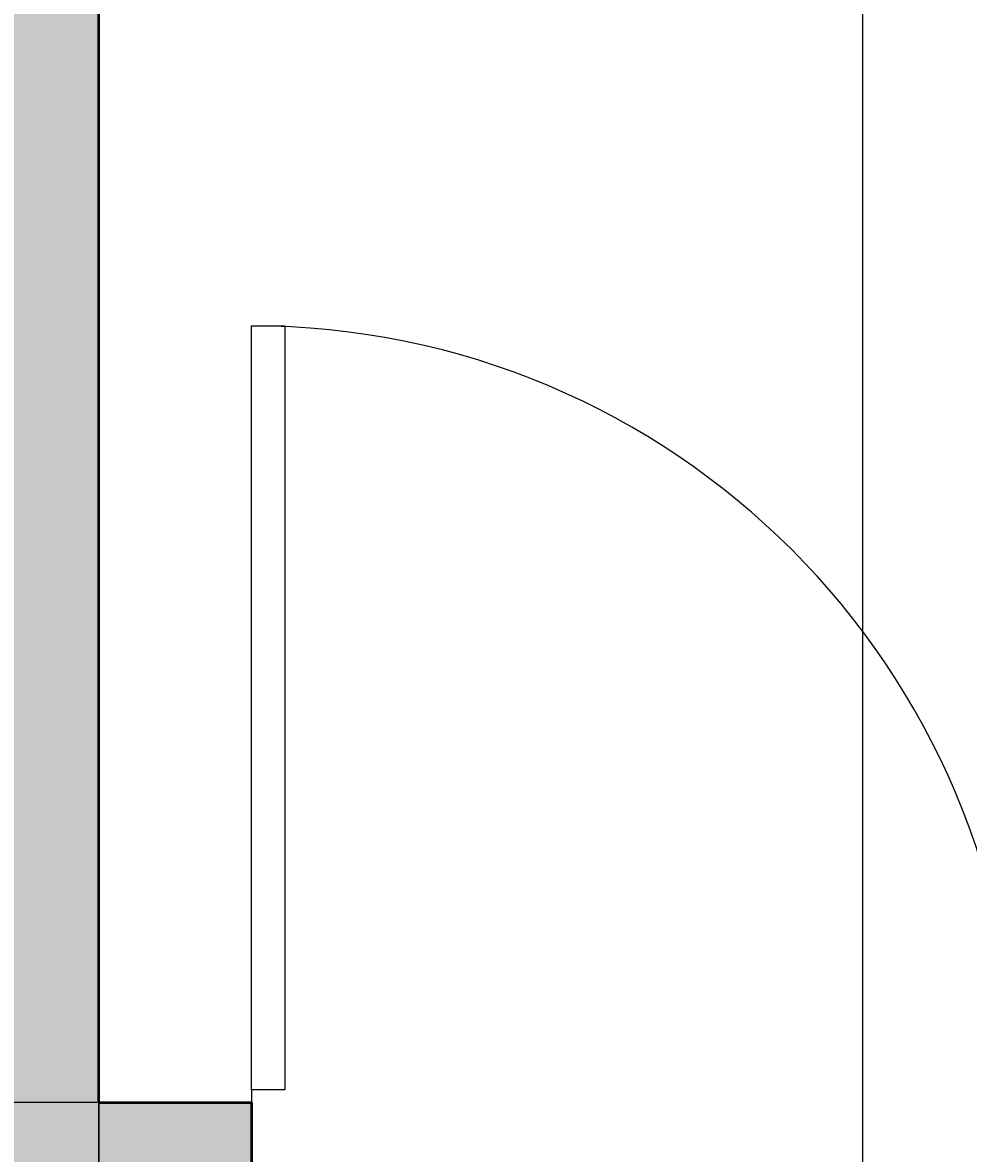
# Model space of a CAD drawing. Units: inches. Extents: x 2307 to 2544, y 2171 to 2540.
# Tile 40 of 52: x 2453 to 2490, y 2438 to 2482. Entities that reach past the tile are written whole.
import ezdxf

# ---------------------------------------------------------------- set-up
doc = ezdxf.new("R2010")
doc.units = ezdxf.units.IN
for name, color, linetype, lineweight in [('A-ANNO-DIMS', 2, 'Continuous', 18), ('A-DOOR', 3, 'Continuous', 25), ('A-WALL', 7, 'Continuous', 50)]:
    doc.layers.add(name, color=color, linetype=linetype, lineweight=lineweight)
doc.layers.add('A-WALL-PATT', color=18, linetype='Continuous', lineweight=13, true_color=0x000000)
doc.styles.get("Standard").update_dxf_attribs({"font": 'arial.ttf'})
doc.dimstyles.get("Standard").update_dxf_attribs({"dimtxt": 0.18, "dimasz": 0.18, "dimexe": 0.18, "dimexo": 0.0625, "dimgap": 0.09, "dimtad": 0, "dimtih": 1, "dimtoh": 1, "dimdec": 4, "dimzin": 0, "dimdsep": 46, "dimtxsty": 'Standard', "dimcen": 0.09, "dimadec": 0, "dimazin": 0, "dimtfac": 1, "dimtdec": 4, "dimtofl": 0, "dimtmove": 0, "dimatfit": 3, "dimfxl": 1, "dimtolj": 1, "dimtzin": 0, "dimarcsym": 0})

# ---------------------------------------------------------------- blocks, each defined once
blk = doc.blocks.new('*U13')
for p, q in [((0, 0), (0, -6)), ((40, 0), (40, -6))]:
    blk.add_line(p, q)
blk.add_lwpolyline([(0, 0), (0, 40), (1.75, 40), (1.75, 0)], close=True)
blk.add_arc((0, 0), 40, 0, 90)
blk = doc.blocks.new('*D48')
at = {"layer": 'A-ANNO-DIMS', "color": 0, "lineweight": -2, "transparency": 16777216}
for p, q in [((2455.633, 2511.51), (2307.366, 2511.51)), ((2307.546, 2511.33), (2307.546, 2475.69)), ((2307.546, 2439.69), (2307.546, 2475.329)), ((2455.633, 2439.51), (2307.366, 2439.51))]:
    blk.add_line(p, q, dxfattribs=at)
at = {"layer": 'A-ANNO-DIMS', "color": 0, "transparency": 16777216}
for points in [[(2307.516, 2511.33), (2307.576, 2511.33), (2307.546, 2511.51)], [(2307.516, 2439.69), (2307.576, 2439.69), (2307.546, 2439.51)]]:
    blk.add_solid(points, dxfattribs=at)
at = {"layer": 'Defpoints', "color": 0, "transparency": 16777216}
for p in [(2307.546, 2511.51), (2455.696, 2511.51), (2455.696, 2439.51)]:
    blk.add_point(p, dxfattribs=at)
at = {"layer": 'A-ANNO-DIMS', "color": 0, "transparency": 16777216, "insert": (2307.546, 2475.51), "char_height": 0.18, "attachment_point": 5}
blk.add_mtext('\\A1;72', dxfattribs=at)
blk = doc.blocks.new('*D53')
at = {"layer": 'A-ANNO-DIMS', "color": 0, "lineweight": -2, "transparency": 16777216}
for p, q in [((2455.696, 2439.447), (2455.696, 2171.18)), ((2461.696, 2439.447), (2461.696, 2171.18)), ((2455.876, 2171.36), (2458.546, 2171.36)), ((2461.516, 2171.36), (2458.845, 2171.36))]:
    blk.add_line(p, q, dxfattribs=at)
at = {"layer": 'A-ANNO-DIMS', "color": 0, "transparency": 16777216}
for points in [[(2455.876, 2171.39), (2455.876, 2171.33), (2455.696, 2171.36)], [(2461.516, 2171.39), (2461.516, 2171.33), (2461.696, 2171.36)]]:
    blk.add_solid(points, dxfattribs=at)
at = {"layer": 'Defpoints', "color": 0, "transparency": 16777216}
for p in [(2455.696, 2439.51), (2461.696, 2439.51), (2461.696, 2171.36)]:
    blk.add_point(p, dxfattribs=at)
at = {"layer": 'A-ANNO-DIMS', "color": 0, "transparency": 16777216, "insert": (2458.696, 2171.36), "char_height": 0.18, "attachment_point": 5}
blk.add_mtext('\\A1;6', dxfattribs=at)
blk = doc.blocks.new('*D59')
at = {"layer": 'A-ANNO-DIMS', "color": 0, "lineweight": -2, "transparency": 16777216}
for p, q in [((2455.696, 2315.572), (2455.696, 2540.345)), ((2455.876, 2540.165), (2470.477, 2540.165)), ((2485.516, 2540.165), (2470.914, 2540.165)), ((2485.696, 2315.572), (2485.696, 2540.345))]:
    blk.add_line(p, q, dxfattribs=at)
at = {"layer": 'A-ANNO-DIMS', "color": 0, "transparency": 16777216}
for points in [[(2455.876, 2540.195), (2455.876, 2540.135), (2455.696, 2540.165)], [(2485.516, 2540.195), (2485.516, 2540.135), (2485.696, 2540.165)]]:
    blk.add_solid(points, dxfattribs=at)
at = {"layer": 'Defpoints', "color": 0, "transparency": 16777216}
for p in [(2455.696, 2540.165), (2455.696, 2315.51), (2485.696, 2315.51)]:
    blk.add_point(p, dxfattribs=at)
at = {"layer": 'A-ANNO-DIMS', "color": 0, "transparency": 16777216, "insert": (2470.696, 2540.165), "char_height": 0.18, "attachment_point": 5}
blk.add_mtext('\\A1;30', dxfattribs=at)

msp = doc.modelspace()

# ---------------------------------------------------------------- hatches: boundary and pattern name
at = {"layer": 'A-WALL-PATT'}
h = msp.add_hatch(color=256, dxfattribs=at)
h.dxf.hatch_style = 1
h.paths.add_polyline_path([(2433.6935, 2199.5096), (2415.6423, 2199.5096), (2415.6423, 2190.5096), (2433.7832, 2190.5096)], flags=17)
h.paths.add_polyline_path([(2367.6423, 2199.5096), (2335.6958, 2199.5096), (2335.6958, 2307.3983), (2326.6958, 2307.3983), (2326.6958, 2190.5096), (2367.6423, 2190.5096)])
h.paths.add_polyline_path([(2524.6958, 2520.5096), (2496.7832, 2520.5096), (2496.7832, 2515.5149), (2472.7832, 2515.5149), (2472.7832, 2520.5096), (2415.4028, 2520.5096), (2415.4028, 2511.5096), (2451.6958, 2511.5096), (2451.6958, 2439.5096), (2451.6958, 2391.5096), (2445.6958, 2391.5096), (2445.6958, 2387.5096), (2455.6958, 2387.5096), (2455.6958, 2435.5096), (2461.6958, 2435.5096), (2461.6958, 2439.5096), (2455.6958, 2439.5096), (2455.6958, 2511.5096), (2515.6958, 2511.5096), (2515.6958, 2439.5096), (2491.6958, 2439.5096), (2491.6958, 2435.5096), (2515.6958, 2435.5096), (2515.6958, 2319.5096), (2451.6958, 2319.5096), (2451.6958, 2281.5096), (2481.6958, 2281.5096), (2481.6958, 2225.5096), (2485.6958, 2225.5096), (2485.6958, 2285.5096), (2455.6958, 2285.5096), (2455.6958, 2315.5096), (2515.6958, 2315.5096), (2515.6958, 2199.5096), (2469.6952, 2199.5096), (2469.785, 2190.5096), (2524.6958, 2190.5096)])

# ---------------------------------------------------------------- linework, layer by layer
at = {"layer": 'A-WALL'}
for p, q in [((2455.6958, 2439.5096), (2455.6958, 2511.5096)), ((2455.6958, 2439.5096), (2461.6958, 2439.5096)), ((2461.6958, 2439.5096), (2461.6958, 2435.5096))]:
    msp.add_line(p, q, dxfattribs=at)

# ---------------------------------------------------------------- block references
at = {"layer": 'A-DOOR', "xscale": 0.75, "yscale": 0.75, "zscale": 0.75}
msp.add_blockref('*U13', (2461.6958, 2440.0096), dxfattribs=at)

# ---------------------------------------------------------------- dimensions: what is measured, and where the dimension line sits
at = {"layer": 'A-ANNO-DIMS'}
for base, p1, p2, picture, middle in [((2455.6958, 2540.1649), (2485.6958, 2315.5096), (2455.6958, 2315.5096), '*D59', (2470.6958, 2540.1649)), ((2461.6958, 2171.3596), (2455.6958, 2439.5096), (2461.6958, 2439.5096), '*D53', (2458.6958, 2171.3596))]:
    dim = msp.add_linear_dim(base=base, p1=p1, p2=p2, dimstyle='Standard', override={"dimdec": 0, "dimlfac": 1, "dimrnd": 0, "dimzin": 0, "dimdsep": 46, "dimlunit": 2}, dxfattribs=at)
    dim.commit()
    dim.dimension.update_dxf_attribs({"geometry": picture, "text_midpoint": middle})
dim = msp.add_linear_dim(base=(2307.5458, 2511.5096), p1=(2455.6958, 2439.5096), p2=(2455.6958, 2511.5096), angle=90, dimstyle='Standard', override={"dimdec": 0, "dimlfac": 1, "dimrnd": 0, "dimzin": 0, "dimdsep": 46, "dimlunit": 2}, dxfattribs=at)
dim.commit()
dim.dimension.update_dxf_attribs({"geometry": '*D48', "text_midpoint": (2307.5458, 2475.5096)})

doc.saveas('drawing.dxf')
